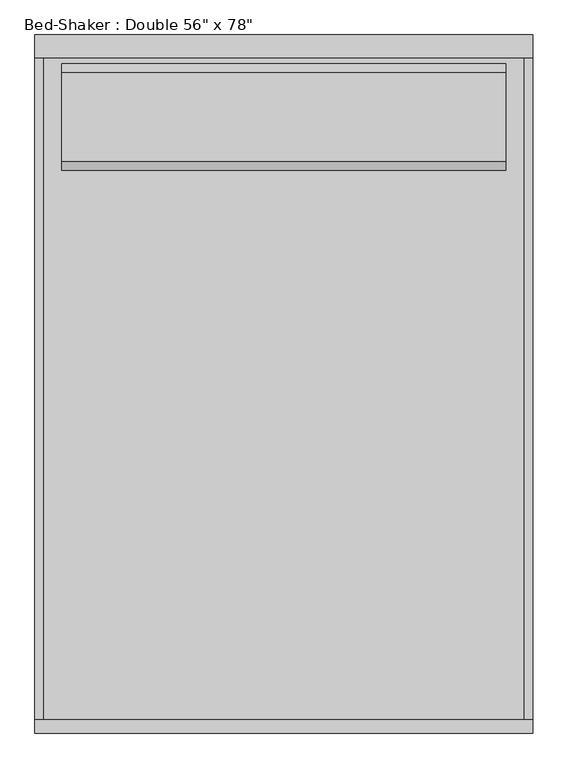
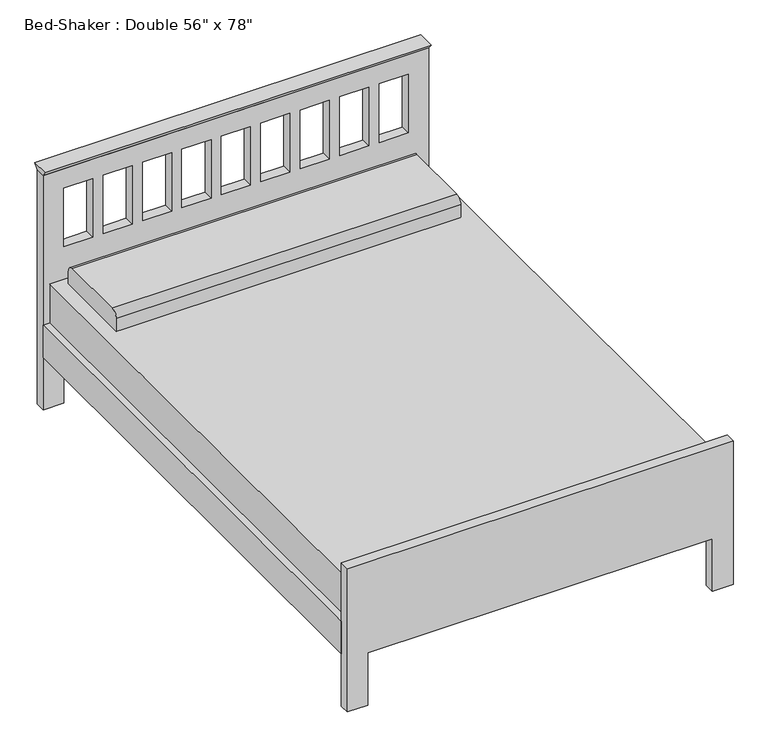
"""IFC4 building model written with IfcOpenShell, lengths in millimetres: furniture geometry."""

from ifc_helpers import new_model, si_unit, point, frame, frame_2d, origin, place, context, project, spatial, polyline, circle_curve, trimmed, segment, composite_curve, outline, extrude, source, transform, mapped, element, save


def furniture_096e7f55(model_context):
    return source(origin(), model_context, "Body", "SweptSolid", [
        extrude(outline(polyline([(-38.1, 914.4), (-51.9545455, 933.45), (13.8545455, 933.45), (0.0, 914.4), (-38.1, 914.4)])), frame((-730.0365546, 0.0, 0.0), z_axis=(1.0, 0.0, 0.0), x_axis=(0.0, 1.0, 0.0)), (0.0, 0.0, 1.0), 1422.4533613),
        extrude(outline(composite_curve([segment(polyline([(-373.2486637, 482.6), (-373.2486637, 533.4)]), True, "CONTINUOUS"), segment(trimmed(circle_curve(frame_2d((-347.8486637, 533.4)), 25.4), [point((-373.2486637, 533.4))], [point((-347.8486637, 558.8))], False, "CARTESIAN"), True, "CONTINUOUS"), segment(polyline([(-347.8486637, 558.8), (-93.8486637, 558.8)]), True, "CONTINUOUS"), segment(trimmed(circle_curve(frame_2d((-93.8486637, 533.4)), 25.4), [point((-93.8486637, 558.8))], [point((-68.4486637, 533.4))], False, "CARTESIAN"), True, "CONTINUOUS"), segment(polyline([(-68.4486637, 533.4), (-68.4486637, 482.6), (-373.2486637, 482.6)]), True, "CONTINUOUS")], self_intersect=False)), frame((-654.05, 0.0, 0.0), z_axis=(1.0, 0.0, 0.0), x_axis=(0.0, 1.0, 0.0)), (0.0, 0.0, 1.0), 1270.0),
        extrude(outline(polyline([(666.75, -38.1), (666.75, -1943.1), (-704.85, -1943.1), (-704.85, -38.1), (666.75, -38.1)])), frame((0.0, 0.0, 228.6), z_axis=(0.0, 0.0, 1.0), x_axis=(1.0, 0.0, 0.0)), (0.0, 0.0, 1.0), 254.0),
        extrude(outline(polyline([(666.75, -1943.1), (666.75, -38.1), (692.15, -38.1), (692.15, -1943.1), (666.75, -1943.1)])), frame((0.0, 0.0, 203.0994861), z_axis=(0.0, 0.0, 1.0), x_axis=(1.0, 0.0, 0.0)), (0.0, 0.0, 1.0), 127.0),
        extrude(outline(polyline([(-730.25, -1943.1), (-730.25, -38.1), (-704.85, -38.1), (-704.85, -1943.1), (-730.25, -1943.1)])), frame((0.0, 0.0, 203.5755296), z_axis=(0.0, 0.0, 1.0), x_axis=(1.0, 0.0, 0.0)), (0.0, 0.0, 1.0), 127.0),
        extrude(outline(polyline([(0.0, -654.05), (203.2, -654.05), (203.2, 615.95), (0.0, 615.95), (0.0, 692.15), (558.8, 692.15), (558.8, -730.25), (0.0, -730.25), (0.0, -654.05)])), frame((0.0, -1981.2, 0.0), z_axis=(0.0, 1.0, 0.0), x_axis=(0.0, 0.0, 1.0)), (0.0, 0.0, 1.0), 38.1),
        extrude(outline(polyline([(914.4, 692.4168067), (914.4, -730.0365546), (0.0, -730.0365546), (0.0, -654.05), (203.2, -654.05), (203.2, 615.95), (0.0, 615.95), (0.0, 692.4168067), (914.4, 692.4168067)]), holes=[polyline([(838.2, -546.8055556), (609.6, -546.8055556), (609.6, -654.05), (838.2, -654.05), (838.2, -546.8055556)]), polyline([(838.2, -401.4611111), (609.6, -401.4611111), (609.6, -508.7055556), (838.2, -508.7055556), (838.2, -401.4611111)]), polyline([(838.2, -256.1166667), (609.6, -256.1166667), (609.6, -363.3611111), (838.2, -363.3611111), (838.2, -256.1166667)]), polyline([(838.2, -110.7722222), (609.6, -110.7722222), (609.6, -218.0166667), (838.2, -218.0166667), (838.2, -110.7722222)]), polyline([(838.2, 179.9166667), (609.6, 179.9166667), (609.6, 72.6722222), (838.2, 72.6722222), (838.2, 179.9166667)]), polyline([(838.2, 325.2611111), (609.6, 325.2611111), (609.6, 218.0166667), (838.2, 218.0166667), (838.2, 325.2611111)]), polyline([(838.2, 470.6055556), (609.6, 470.6055556), (609.6, 363.3611111), (838.2, 363.3611111), (838.2, 470.6055556)]), polyline([(838.2, 615.95), (609.6, 615.95), (609.6, 508.7055556), (838.2, 508.7055556), (838.2, 615.95)]), polyline([(838.2, 34.5722222), (609.6, 34.5722222), (609.6, -72.6722222), (838.2, -72.6722222), (838.2, 34.5722222)])]), frame((0.0, -38.1, 0.0), z_axis=(0.0, 1.0, 0.0), x_axis=(0.0, 0.0, 1.0)), (0.0, 0.0, 1.0), 38.1),
    ])


if __name__ == "__main__":
    model = new_model("IFC4")
    model_context = context("Model", 3, world=origin())
    ifc_project = project(units=[si_unit("LENGTHUNIT", "METRE", prefix="MILLI")], contexts=[model_context])
    site = spatial("IfcSite", under=ifc_project)
    building = spatial("IfcBuilding", under=site)
    placement = place(None, origin())
    furniture_shape = furniture_096e7f55(model_context)
    element("IfcFurniture", 1, ObjectType="Bed-Shaker : Double 56\" x 78\"", at=placement, inside=building, context=model_context, shape_type="MappedRepresentation", body=[
        mapped(furniture_shape, transform((0.0, 0.0, 0.0), x_axis=(1.0, 0.0, 0.0), y_axis=(0.0, 1.0, 0.0), z_axis=(0.0, 0.0, 1.0))),
    ])
    save(model, "model.ifc")

# Revit data of these elements
# Type "Bed-Shaker : Double 56\" x 78\""
#   Assembly Code = "E2020200"
#   Length = 6' - 6"
#   Width = 4' - 8"
#   Frame Material = Birch
#   Mattress Material = Softwood, Lumber
#   Default Elevation = 0
# Element 1 (IfcFurniture, "Bed-Shaker : Double 56\" x 78\"")
#   Materials on its faces: "Birch", "Softwood, Lumber"
# Materials
#   "Birch": class "Wood", colour RGB 224 178 126, transparency 0, Description = "Betula Alleghaniensis", Cost = 0
#   "Softwood, Lumber": class "Wood", colour RGB 223 192 134, transparency 0, Description = "Pinus Echinata", Cost = 0
